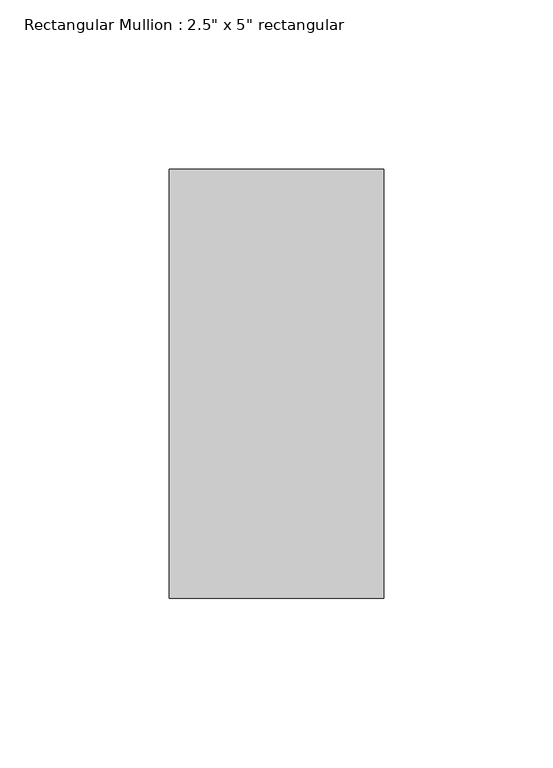
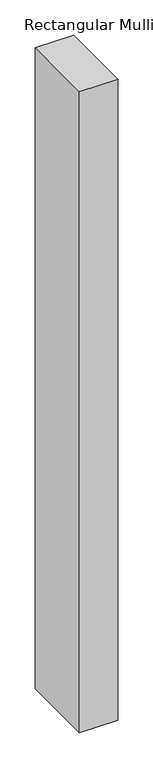
"""IFC4 building model written with IfcOpenShell, lengths in millimetres: member geometry."""

from ifc_helpers import new_model, si_unit, frame, origin, place, context, project, spatial, polyline, outline, extrude, source, transform, mapped, element, save


def member_211d5d53(model_context):
    return source(origin(), model_context, "Body", "SweptSolid", [
        extrude(outline(polyline([(0.0, 63.5), (0.0, -63.5), (-63.5, -63.5), (-63.5, 63.5), (0.0, 63.5)])), frame((0.0, 0.0, -1117.5999998), z_axis=(0.0, 0.0, 1.0), x_axis=(1.0, 0.0, 0.0)), (0.0, 0.0, 1.0), 1117.5999998),
    ])


if __name__ == "__main__":
    model = new_model("IFC4")
    model_context = context("Model", 3, world=origin())
    ifc_project = project(units=[si_unit("LENGTHUNIT", "METRE", prefix="MILLI")], contexts=[model_context])
    site = spatial("IfcSite", under=ifc_project)
    building = spatial("IfcBuilding", under=site)
    placement = place(None, origin())
    member_shape = member_211d5d53(model_context)
    element("IfcMember", 1, ObjectType="Rectangular Mullion : 2.5\" x 5\" rectangular", at=placement, inside=building, context=model_context, shape_type="MappedRepresentation", body=[
        mapped(member_shape, transform((0.0, 0.0, 0.0), x_axis=(1.0, 0.0, 0.0), y_axis=(0.0, 1.0, 0.0), z_axis=(0.0, 0.0, 1.0))),
    ])
    save(model, "model.ifc")

# Revit data of these elements
# Type "Rectangular Mullion : 2.5\" x 5\" rectangular"
#   built-in parameter 1007304 = 0.416667 (stored number, unit not read)
#   built-in parameter 1007301 = 0.104167 (stored number, unit not read)
#   built-in parameter 1007300 = 0.104167 (stored number, unit not read)
# Element 1 (IfcMember, "Rectangular Mullion : 2.5\" x 5\" rectangular")
#   Materials on its faces: "Aluminum"
# Materials
#   "Aluminum": class "Metal", colour RGB 247 247 247, transparency 0, Description = "Aluminum 6061", Cost = 0
